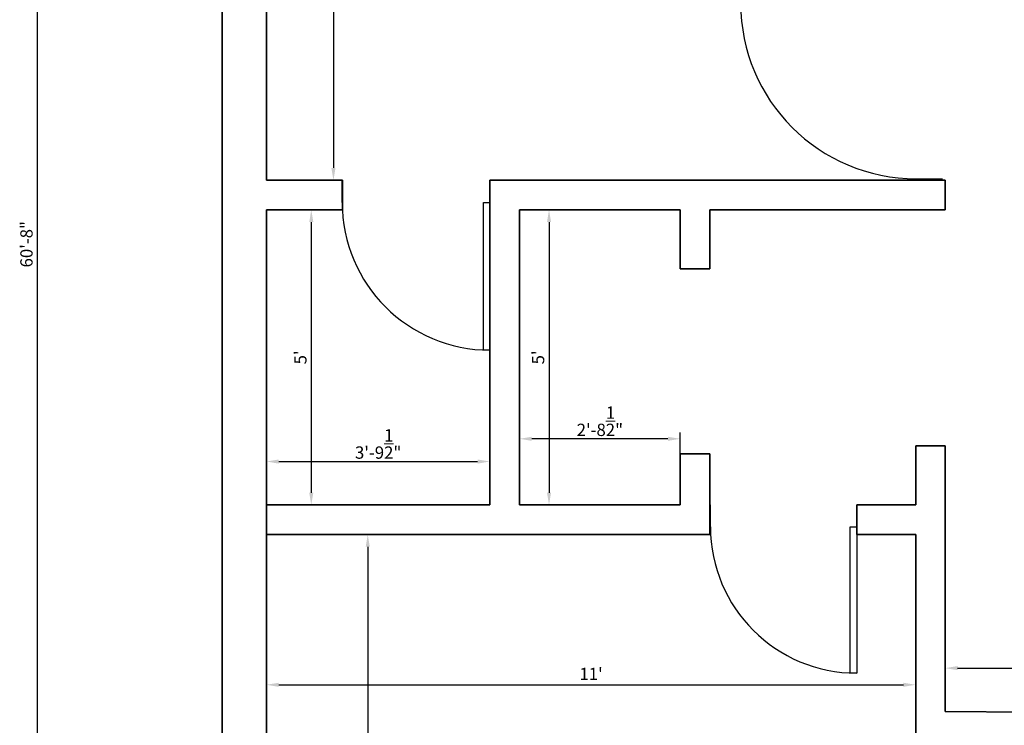
# Model space of a CAD drawing. Units: inches. Extents: x 2025 to 2528, y 1525 to 2336.
# Tile 5 of 18: x 2025 to 2225, y 1831 to 1974. Entities that reach past the tile are written whole.
import ezdxf

# ---------------------------------------------------------------- set-up
doc = ezdxf.new("R2010")
doc.units = ezdxf.units.IN
for name, color, linetype, lineweight in [('A-ANNO-DIMS', 2, 'Continuous', 18), ('A-DOOR', 3, 'Continuous', 25), ('A-WALL', 7, 'Continuous', 35)]:
    doc.layers.add(name, color=color, linetype=linetype, lineweight=lineweight)
doc.styles.get("Standard").update_dxf_attribs({"font": 'arial.ttf'})
doc.dimstyles.new('Copy of ISO-25', dxfattribs={"dimtxt": 2.5, "dimasz": 2.5, "dimexe": 1.25, "dimexo": 0.625, "dimtad": 1, "dimdec": 1, "dimlunit": 4, "dimtxsty": 'Standard', "dimcen": 2.5, "dimadec": 0, "dimazin": 0, "dimtfac": 1, "dimtdec": 1, "dimtmove": 0, "dimatfit": 3, "dimfxl": 1, "dimarcsym": 0})

# ---------------------------------------------------------------- blocks, each defined once
blk = doc.blocks.new('*U5')
for p, q in [((0, 0), (0, -6)), ((-40, 0), (-40, -6))]:
    blk.add_line(p, q)
blk.add_lwpolyline([(0, 0), (0, 40), (-1.75, 40), (-1.75, 0)], close=True)
blk.add_arc((0, 0), 40, 90, 180)
blk = doc.blocks.new('*U4')
for p, q in [((-40, 0), (-40, 6)), ((0, 0), (0, 6))]:
    blk.add_line(p, q)
blk.add_lwpolyline([(0, 0), (0, -40), (-1.75, -40), (-1.75, 0)], close=True)
blk.add_arc((0, 0), 40, 180, 270)
blk = doc.blocks.new('*D13')
at = {"layer": 'A-ANNO-DIMS', "color": 0, "lineweight": -2, "transparency": 16777216}
for p, q in [((2075.64, 2109.41), (2089.89, 2109.41)), ((2088.64, 2106.91), (2088.64, 1943.91)), ((2075.64, 1941.41), (2089.89, 1941.41))]:
    blk.add_line(p, q, dxfattribs=at)
at = {"layer": 'A-ANNO-DIMS', "color": 0, "transparency": 16777216}
for points in [[(2088.22, 2106.91), (2089.06, 2106.91), (2088.64, 2109.41)], [(2088.22, 1943.91), (2089.06, 1943.91), (2088.64, 1941.41)]]:
    blk.add_solid(points, dxfattribs=at)
at = {"layer": 'Defpoints', "color": 0, "transparency": 16777216}
for p in [(2075.01, 2109.41), (2075.01, 1941.41), (2088.64, 1941.41)]:
    blk.add_point(p, dxfattribs=at)
at = {"layer": 'A-ANNO-DIMS', "color": 0, "transparency": 16777216, "insert": (2086.76, 2025.41), "char_height": 2.5, "attachment_point": 5, "rotation": 90}
blk.add_mtext("14'", dxfattribs=at)
blk = doc.blocks.new('*D25')
at = {"layer": 'A-ANNO-DIMS', "color": 0, "lineweight": -2, "transparency": 16777216}
for p, q in [((2075.01, 1876.04), (2075.01, 1885.49)), ((2120.45, 1876.04), (2120.45, 1885.49)), ((2077.51, 1884.24), (2117.95, 1884.24))]:
    blk.add_line(p, q, dxfattribs=at)
at = {"layer": 'A-ANNO-DIMS', "color": 0, "transparency": 16777216}
for points in [[(2077.51, 1884.65), (2077.51, 1883.82), (2075.01, 1884.24)], [(2117.95, 1884.65), (2117.95, 1883.82), (2120.45, 1884.24)]]:
    blk.add_solid(points, dxfattribs=at)
at = {"layer": 'Defpoints', "color": 0, "transparency": 16777216}
for p in [(2120.45, 1884.24), (2075.01, 1875.41), (2120.45, 1875.41)]:
    blk.add_point(p, dxfattribs=at)
at = {"layer": 'A-ANNO-DIMS', "color": 0, "transparency": 16777216, "insert": (2097.73, 1887.81), "char_height": 2.5, "attachment_point": 5}
blk.add_mtext('3\'-9{\\H1x;\\S1/2;}"', dxfattribs=at)
blk = doc.blocks.new('*D26')
at = {"layer": 'A-ANNO-DIMS', "color": 0, "lineweight": -2, "transparency": 16777216}
for p, q in [((2075.64, 1935.41), (2085.38, 1935.41)), ((2084.13, 1932.91), (2084.13, 1877.91)), ((2075.64, 1875.41), (2085.38, 1875.41))]:
    blk.add_line(p, q, dxfattribs=at)
at = {"layer": 'A-ANNO-DIMS', "color": 0, "transparency": 16777216}
for points in [[(2083.72, 1932.91), (2084.55, 1932.91), (2084.13, 1935.41)], [(2083.72, 1877.91), (2084.55, 1877.91), (2084.13, 1875.41)]]:
    blk.add_solid(points, dxfattribs=at)
at = {"layer": 'Defpoints', "color": 0, "transparency": 16777216}
for p in [(2075.01, 1935.41), (2075.01, 1875.41), (2084.13, 1875.41)]:
    blk.add_point(p, dxfattribs=at)
at = {"layer": 'A-ANNO-DIMS', "color": 0, "transparency": 16777216, "insert": (2082.24, 1905.41), "char_height": 2.5, "attachment_point": 5, "rotation": 90}
blk.add_mtext("5'", dxfattribs=at)
blk = doc.blocks.new('*D27')
at = {"layer": 'A-ANNO-DIMS', "color": 0, "lineweight": -2, "transparency": 16777216}
for p, q in [((2126.45, 1876.04), (2126.45, 1890.11)), ((2159.14, 1876.04), (2159.14, 1890.11)), ((2156.64, 1888.86), (2128.95, 1888.86))]:
    blk.add_line(p, q, dxfattribs=at)
at = {"layer": 'A-ANNO-DIMS', "color": 0, "transparency": 16777216}
for points in [[(2128.95, 1889.27), (2128.95, 1888.44), (2126.45, 1888.86)], [(2156.64, 1889.27), (2156.64, 1888.44), (2159.14, 1888.86)]]:
    blk.add_solid(points, dxfattribs=at)
at = {"layer": 'Defpoints', "color": 0, "transparency": 16777216}
for p in [(2126.45, 1888.86), (2126.45, 1875.41), (2159.14, 1875.41)]:
    blk.add_point(p, dxfattribs=at)
at = {"layer": 'A-ANNO-DIMS', "color": 0, "transparency": 16777216, "insert": (2142.8, 1892.43), "char_height": 2.5, "attachment_point": 5}
blk.add_mtext('2\'-8{\\H1x;\\S1/2;}"', dxfattribs=at)
blk = doc.blocks.new('*D28')
at = {"layer": 'A-ANNO-DIMS', "color": 0, "lineweight": -2, "transparency": 16777216}
for p, q in [((2127.08, 1935.41), (2133.71, 1935.41)), ((2132.46, 1932.91), (2132.46, 1877.91)), ((2127.08, 1875.41), (2133.71, 1875.41))]:
    blk.add_line(p, q, dxfattribs=at)
at = {"layer": 'A-ANNO-DIMS', "color": 0, "transparency": 16777216}
for points in [[(2132.05, 1932.91), (2132.88, 1932.91), (2132.46, 1935.41)], [(2132.05, 1877.91), (2132.88, 1877.91), (2132.46, 1875.41)]]:
    blk.add_solid(points, dxfattribs=at)
at = {"layer": 'Defpoints', "color": 0, "transparency": 16777216}
for p in [(2126.45, 1935.41), (2126.45, 1875.41), (2132.46, 1875.41)]:
    blk.add_point(p, dxfattribs=at)
at = {"layer": 'A-ANNO-DIMS', "color": 0, "transparency": 16777216, "insert": (2130.57, 1905.41), "char_height": 2.5, "attachment_point": 5, "rotation": 90}
blk.add_mtext("5'", dxfattribs=at)
blk = doc.blocks.new('*D29')
at = {"layer": 'A-ANNO-DIMS', "color": 0, "lineweight": -2, "transparency": 16777216}
for p, q in [((2075.01, 1868.79), (2075.01, 1837.61)), ((2207.01, 1868.79), (2207.01, 1837.61)), ((2077.51, 1838.86), (2204.51, 1838.86))]:
    blk.add_line(p, q, dxfattribs=at)
at = {"layer": 'A-ANNO-DIMS', "color": 0, "transparency": 16777216}
for points in [[(2077.51, 1839.27), (2077.51, 1838.44), (2075.01, 1838.86)], [(2204.51, 1839.27), (2204.51, 1838.44), (2207.01, 1838.86)]]:
    blk.add_solid(points, dxfattribs=at)
at = {"layer": 'Defpoints', "color": 0, "transparency": 16777216}
for p in [(2075.01, 1869.41), (2207.01, 1869.41), (2207.01, 1838.86)]:
    blk.add_point(p, dxfattribs=at)
at = {"layer": 'A-ANNO-DIMS', "color": 0, "transparency": 16777216, "insert": (2141.01, 1840.74), "char_height": 2.5, "attachment_point": 5}
blk.add_mtext("11'", dxfattribs=at)
blk = doc.blocks.new('*D30')
at = {"layer": 'A-ANNO-DIMS', "color": 0, "lineweight": -2, "transparency": 16777216}
for p, q in [((2078.14, 1869.41), (2096.86, 1869.41)), ((2095.61, 1866.91), (2095.61, 1715.91)), ((2075.64, 1713.41), (2096.86, 1713.41))]:
    blk.add_line(p, q, dxfattribs=at)
at = {"layer": 'A-ANNO-DIMS', "color": 0, "transparency": 16777216}
for points in [[(2095.2, 1866.91), (2096.03, 1866.91), (2095.61, 1869.41)], [(2095.2, 1715.91), (2096.03, 1715.91), (2095.61, 1713.41)]]:
    blk.add_solid(points, dxfattribs=at)
at = {"layer": 'Defpoints', "color": 0, "transparency": 16777216}
for p in [(2077.51, 1869.41), (2075.01, 1713.41), (2095.61, 1713.41)]:
    blk.add_point(p, dxfattribs=at)
at = {"layer": 'A-ANNO-DIMS', "color": 0, "transparency": 16777216, "insert": (2093.71, 1791.41), "char_height": 2.5, "attachment_point": 5, "rotation": 90}
blk.add_mtext("13'", dxfattribs=at)
blk = doc.blocks.new('*D35')
at = {"layer": 'A-ANNO-DIMS', "color": 0, "lineweight": -2, "transparency": 16777216}
for p, q in [((2213.01, 1834.04), (2213.01, 1843.49)), ((2254.78, 1833.8), (2254.78, 1843.49)), ((2215.51, 1842.24), (2252.28, 1842.24))]:
    blk.add_line(p, q, dxfattribs=at)
at = {"layer": 'A-ANNO-DIMS', "color": 0, "transparency": 16777216}
for points in [[(2215.51, 1842.66), (2215.51, 1841.83), (2213.01, 1842.24)], [(2252.28, 1842.66), (2252.28, 1841.83), (2254.78, 1842.24)]]:
    blk.add_solid(points, dxfattribs=at)
at = {"layer": 'Defpoints', "color": 0, "transparency": 16777216}
for p in [(2254.78, 1842.24), (2213.01, 1833.41), (2254.78, 1833.18)]:
    blk.add_point(p, dxfattribs=at)
at = {"layer": 'A-ANNO-DIMS', "color": 0, "transparency": 16777216, "insert": (2233.89, 1844.15), "char_height": 2.5, "attachment_point": 5}
blk.add_mtext('3\'-6"', dxfattribs=at)
blk = doc.blocks.new('*D80')
at = {"layer": 'A-ANNO-DIMS', "color": 0, "lineweight": -2, "transparency": 16777216}
for p, q in [((2065.39, 2292.41), (2027.21, 2292.41)), ((2028.46, 1566.91), (2028.46, 2289.91)), ((2285.39, 1564.41), (2027.21, 1564.41))]:
    blk.add_line(p, q, dxfattribs=at)
at = {"layer": 'A-ANNO-DIMS', "color": 0, "transparency": 16777216}
for points in [[(2028.05, 2289.91), (2028.88, 2289.91), (2028.46, 2292.41)], [(2028.05, 1566.91), (2028.88, 1566.91), (2028.46, 1564.41)]]:
    blk.add_solid(points, dxfattribs=at)
at = {"layer": 'Defpoints', "color": 0, "transparency": 16777216}
for p in [(2028.46, 2292.41), (2066.01, 2292.41), (2286.01, 1564.41)]:
    blk.add_point(p, dxfattribs=at)
at = {"layer": 'A-ANNO-DIMS', "color": 0, "transparency": 16777216, "insert": (2026.56, 1928.41), "char_height": 2.5, "attachment_point": 5, "rotation": 90}
blk.add_mtext('60\'-8"', dxfattribs=at)

msp = doc.modelspace()

# ---------------------------------------------------------------- linework, layer by layer
at = {"layer": 'A-WALL'}
for p, q in [((2066.01, 2109.41), (2066.01, 1941.41)), ((2075.01, 2109.41), (2075.01, 1941.41)), ((2066.01, 1941.41), (2066.01, 1935.41)), ((2075.01, 1941.41), (2090.45, 1941.41)), ((2075.01, 1941.41), (2090.45, 1941.41)), ((2090.45, 1941.41), (2090.45, 1935.41)), ((2120.45, 1935.41), (2120.45, 1941.41)), ((2120.45, 1941.41), (2138.45, 1941.41)), ((2138.45, 1941.41), (2165.14, 1941.41)), ((2213.01, 1941.41), (2165.14, 1941.41)), ((2213.01, 1935.41), (2213.01, 1941.41)), ((2066.01, 1935.41), (2066.01, 1887.41)), ((2075.01, 1935.41), (2075.01, 1887.41)), ((2090.45, 1935.41), (2075.01, 1935.41)), ((2120.45, 1935.41), (2120.45, 1875.41)), ((2126.45, 1935.41), (2138.45, 1935.41)), ((2126.45, 1875.41), (2126.45, 1935.41)), ((2159.14, 1935.41), (2138.45, 1935.41)), ((2159.14, 1935.41), (2159.14, 1923.41)), ((2159.14, 1935.41), (2159.14, 1923.41)), ((2165.14, 1935.41), (2213.01, 1935.41)), ((2165.14, 1923.41), (2165.14, 1935.41)), ((2159.14, 1923.41), (2165.14, 1923.41)), ((2066.01, 1887.41), (2066.01, 1881.41)), ((2075.01, 1887.41), (2075.01, 1881.41)), ((2159.14, 1875.41), (2159.14, 1885.81)), ((2159.14, 1885.81), (2165.14, 1885.81)), ((2159.14, 1885.81), (2159.14, 1875.41)), ((2165.14, 1875.41), (2165.14, 1885.81)), ((2207.01, 1875.41), (2207.01, 1887.41)), ((2213.01, 1887.41), (2207.01, 1887.41)), ((2213.01, 1875.41), (2213.01, 1887.41)), ((2213.01, 1887.41), (2213.01, 1875.41)), ((2066.01, 1881.41), (2066.01, 1713.41)), ((2075.01, 1881.41), (2075.01, 1713.41)), ((2075.01, 1875.41), (2075.01, 1869.41)), ((2120.45, 1875.41), (2075.01, 1875.41)), ((2159.14, 1875.41), (2126.45, 1875.41)), ((2165.14, 1875.41), (2165.14, 1869.41)), ((2207.01, 1875.41), (2195.01, 1875.41)), ((2207.01, 1875.41), (2195.01, 1875.41)), ((2195.01, 1875.41), (2195.01, 1869.41)), ((2213.01, 1875.41), (2213.01, 1875.41)), ((2213.01, 1875.41), (2213.01, 1869.41)), ((2075.01, 1869.41), (2165.14, 1869.41)), ((2195.01, 1869.41), (2207.01, 1869.41)), ((2207.01, 1827.18), (2207.01, 1869.41)), ((2213.01, 1869.41), (2213.01, 1833.41)), ((2213.01, 1833.41), (2254.78, 1833.18))]:
    msp.add_line(p, q, dxfattribs=at)

# ---------------------------------------------------------------- block references
at = {"layer": 'A-DOOR', "xscale": 0.8923728301010077, "yscale": 0.8923728301010077, "zscale": 0.8923728301010077, "rotation": 90}
msp.add_blockref('*U5', (2207.11, 1977.41), dxfattribs=at)
at = {"layer": 'A-DOOR'}
for p, xscale, yscale, zscale in [((2120.45, 1936.91), 0.7506984196359394, 0.7506984196359394, 0.7506984196359394), ((2195.01, 1870.95), 0.7432372337132856, 0.7432372337132856, 0.7432372337132856)]:
    msp.add_blockref('*U4', p, dxfattribs=dict(at, xscale=xscale, yscale=yscale, zscale=zscale))

# ---------------------------------------------------------------- dimensions: what is measured, and where the dimension line sits
at = {"layer": 'A-ANNO-DIMS'}
for base, p1, p2, override, picture, middle in [((2028.46, 2292.41), (2286.01, 1564.41), (2066.01, 2292.41), {"dimdec": 1, "dimlfac": 1, "dimrnd": 0, "dimzin": 1, "dimdsep": 46, "dimlunit": 4, "dimfrac": 2}, '*D80', (2026.56, 1928.41)), ((2088.64, 1941.41), (2075.01, 2109.41), (2075.01, 1941.41), {"dimclrd": 0, "dimclre": 0, "dimclrt": 0}, '*D13', (2086.76, 2025.41)), ((2084.13, 1875.41), (2075.01, 1935.41), (2075.01, 1875.41), {"dimclrd": 0, "dimclre": 0, "dimclrt": 0}, '*D26', (2082.24, 1905.41)), ((2132.46, 1875.41), (2126.45, 1935.41), (2126.45, 1875.41), {"dimclrd": 0, "dimclre": 0, "dimclrt": 0}, '*D28', (2130.57, 1905.41)), ((2095.61, 1713.41), (2077.51, 1869.41), (2075.01, 1713.41), {"dimclrd": 0, "dimclre": 0, "dimclrt": 0}, '*D30', (2093.71, 1791.41))]:
    dim = msp.add_linear_dim(base=base, p1=p1, p2=p2, angle=90, dimstyle='Copy of ISO-25', override=override, dxfattribs=at)
    dim.commit()
    dim.dimension.update_dxf_attribs({"geometry": picture, "text_midpoint": middle})
for base, p1, p2, picture, middle in [((2126.45, 1888.86), (2159.14, 1875.41), (2126.45, 1875.41), '*D27', (2142.8, 1892.43)), ((2120.45, 1884.24), (2075.01, 1875.41), (2120.45, 1875.41), '*D25', (2097.73, 1887.81)), ((2207.01, 1838.86), (2075.01, 1869.41), (2207.01, 1869.41), '*D29', (2141.01, 1840.74)), ((2254.78, 1842.24), (2213.01, 1833.41), (2254.78, 1833.18), '*D35', (2233.89, 1844.15))]:
    dim = msp.add_linear_dim(base=base, p1=p1, p2=p2, dimstyle='Copy of ISO-25', override={"dimclrd": 0, "dimclre": 0, "dimclrt": 0}, dxfattribs=at)
    dim.commit()
    dim.dimension.update_dxf_attribs({"geometry": picture, "text_midpoint": middle})

doc.saveas('drawing.dxf')
